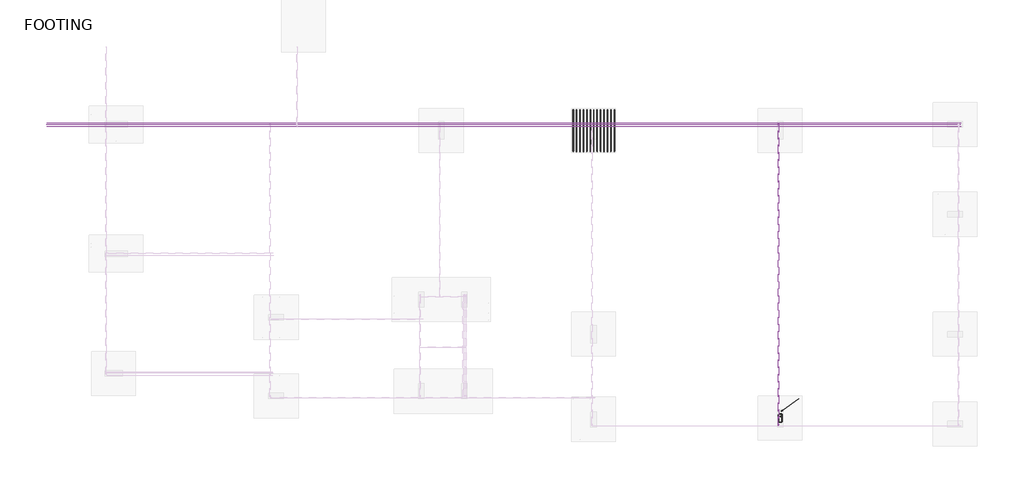
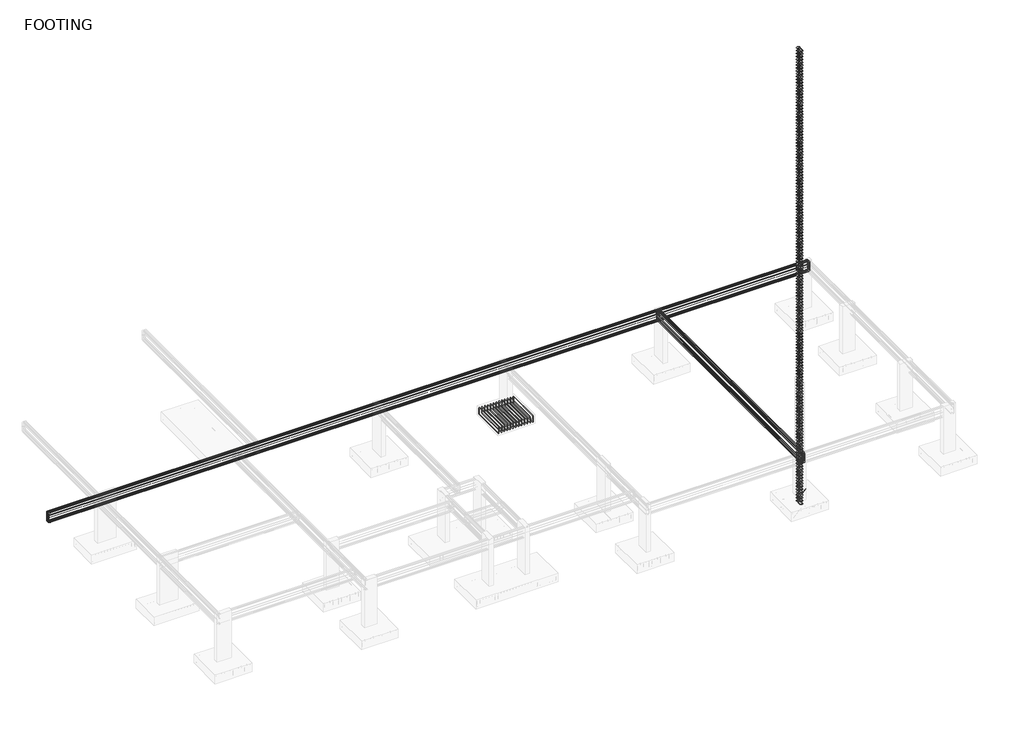
# One storey, part 7 of 12: 10 reinforcing bars.
"""IFC4 building model written with IfcOpenShell, lengths in millimetres."""

from ifc_helpers import new_model, si_unit, point, frame, origin, place, context, project, spatial, polyline, circle_curve, trimmed, segment, composite_curve, source, transform, mapped, element, save
from ifc_brep_helpers import swept_disk

model = new_model("IFC4")

# Units and contexts
model_context = context("Model", 3, world=origin())
ifc_project = project(units=[si_unit("LENGTHUNIT", "METRE", prefix="MILLI")], contexts=[model_context])

# Site, building, storey
site = spatial("IfcSite", under=ifc_project)
building = spatial("IfcBuilding", under=site)
storey = spatial("IfcBuildingStorey", under=building, Name="FOOTING", Elevation=-5638.8)

# Reinforcing bars
placement = place(None, origin())
reinforcing_bar_shape = source(origin(), model_context, "Body", "SolidModel", [
    swept_disk(composite_curve([segment(polyline([(5332.7998335, -3250.2541655, -5788.8), (5332.7998335, -3250.2541655, -5975.4)]), True, "CONTINUOUS"), segment(trimmed(circle_curve(frame((5332.7998335, -3194.8041655, -5975.4), z_axis=(1.0, 0.0, 0.0), x_axis=(0.0, -55.44999999999982, 0.0)), 55.45), [point((5332.7998335, -3250.2541655, -5975.4))], [point((5332.7998335, -3194.8041655, -6030.85))], True, "CARTESIAN"), True, "CONTINUOUS"), segment(polyline([(5332.7998335, -3194.8041655, -6030.85), (5332.7998335, -1621.6041655, -6030.85)]), True, "CONTINUOUS"), segment(trimmed(circle_curve(frame((5332.7998335, -1621.6041655, -5975.4), z_axis=(1.0, 0.0, 0.0), x_axis=(0.0, 0.0, -55.45000000000073)), 55.45), [point((5332.7998335, -1621.6041655, -6030.85))], [point((5332.7998335, -1566.1541655, -5975.4))], True, "CARTESIAN"), True, "CONTINUOUS"), segment(polyline([(5332.7998335, -1566.1541655, -5975.4), (5332.7998335, -1566.1541655, -5788.8)]), True, "CONTINUOUS")], self_intersect=False), 7.95),
])
element("IfcReinforcingBar", 1, at=placement, inside=storey, context=model_context, shape_type="MappedRepresentation", body=[
    mapped(reinforcing_bar_shape, transform((0.0, 0.0, 0.0), x_axis=(1.0, 0.0, 0.0), y_axis=(0.0, 1.0, 0.0), z_axis=(0.0, 0.0, 1.0))),
    mapped(reinforcing_bar_shape, transform((-140.3416667, 0.0, 0.0), x_axis=(1.0, 0.0, 0.0), y_axis=(0.0, 1.0, 0.0), z_axis=(0.0, 0.0, 1.0))),
    mapped(reinforcing_bar_shape, transform((-280.6833333, 0.0, 0.0), x_axis=(1.0, 0.0, 0.0), y_axis=(0.0, 1.0, 0.0), z_axis=(0.0, 0.0, 1.0))),
    mapped(reinforcing_bar_shape, transform((-421.025, 0.0, 0.0), x_axis=(1.0, 0.0, 0.0), y_axis=(0.0, 1.0, 0.0), z_axis=(0.0, 0.0, 1.0))),
    mapped(reinforcing_bar_shape, transform((-561.3666667, 0.0, 0.0), x_axis=(1.0, 0.0, 0.0), y_axis=(0.0, 1.0, 0.0), z_axis=(0.0, 0.0, 1.0))),
    mapped(reinforcing_bar_shape, transform((-701.7083333, 0.0, 0.0), x_axis=(1.0, 0.0, 0.0), y_axis=(0.0, 1.0, 0.0), z_axis=(0.0, 0.0, 1.0))),
    mapped(reinforcing_bar_shape, transform((-842.05, 0.0, 0.0), x_axis=(1.0, 0.0, 0.0), y_axis=(0.0, 1.0, 0.0), z_axis=(0.0, 0.0, 1.0))),
    mapped(reinforcing_bar_shape, transform((-982.3916667, 0.0, 0.0), x_axis=(1.0, 0.0, 0.0), y_axis=(0.0, 1.0, 0.0), z_axis=(0.0, 0.0, 1.0))),
    mapped(reinforcing_bar_shape, transform((-1122.7333333, 0.0, 0.0), x_axis=(1.0, 0.0, 0.0), y_axis=(0.0, 1.0, 0.0), z_axis=(0.0, 0.0, 1.0))),
    mapped(reinforcing_bar_shape, transform((-1263.075, 0.0, 0.0), x_axis=(1.0, 0.0, 0.0), y_axis=(0.0, 1.0, 0.0), z_axis=(0.0, 0.0, 1.0))),
    mapped(reinforcing_bar_shape, transform((-1403.4166667, 0.0, 0.0), x_axis=(1.0, 0.0, 0.0), y_axis=(0.0, 1.0, 0.0), z_axis=(0.0, 0.0, 1.0))),
    mapped(reinforcing_bar_shape, transform((-1543.7583333, 0.0, 0.0), x_axis=(1.0, 0.0, 0.0), y_axis=(0.0, 1.0, 0.0), z_axis=(0.0, 0.0, 1.0))),
    mapped(reinforcing_bar_shape, transform((-1684.1, 0.0, 0.0), x_axis=(1.0, 0.0, 0.0), y_axis=(0.0, 1.0, 0.0), z_axis=(0.0, 0.0, 1.0))),
])
reinforcing_bar_2_shape = source(origin(), model_context, "Body", "SolidModel", [
    swept_disk(composite_curve([segment(polyline([(5323.6597994, -1564.5541655, -5888.8), (5323.6597994, -1564.5541655, -5741.5)]), True, "CONTINUOUS"), segment(trimmed(circle_curve(frame((5323.6597994, -1610.9041655, -5741.5), z_axis=(1.0, 0.0, 0.0), x_axis=(0.0, 46.350000000000136, 0.0)), 46.35), [point((5323.6597994, -1564.5541655, -5741.5))], [point((5323.6597994, -1610.9041655, -5695.15))], True, "CARTESIAN"), True, "CONTINUOUS"), segment(polyline([(5323.6597994, -1610.9041655, -5695.15), (5323.6597994, -3205.5041655, -5695.15)]), True, "CONTINUOUS"), segment(trimmed(circle_curve(frame((5323.6597994, -3205.5041655, -5741.5), z_axis=(1.0, 0.0, 0.0), x_axis=(0.0, 0.0, 46.350000000000364)), 46.35), [point((5323.6597994, -3205.5041655, -5695.15))], [point((5323.6597994, -3251.8541655, -5741.5))], True, "CARTESIAN"), True, "CONTINUOUS"), segment(polyline([(5323.6597994, -3251.8541655, -5741.5), (5323.6597994, -3251.8541655, -5888.8)]), True, "CONTINUOUS")], self_intersect=False), 6.35),
])
element("IfcReinforcingBar", 2, at=placement, inside=storey, context=model_context, shape_type="MappedRepresentation", body=[
    mapped(reinforcing_bar_2_shape, transform((0.0, 0.0, 0.0), x_axis=(1.0, 0.0, 0.0), y_axis=(0.0, 1.0, 0.0), z_axis=(0.0, 0.0, 1.0))),
    mapped(reinforcing_bar_2_shape, transform((-138.4829293, 0.0, 0.0), x_axis=(1.0, 0.0, 0.0), y_axis=(0.0, 1.0, 0.0), z_axis=(0.0, 0.0, 1.0))),
    mapped(reinforcing_bar_2_shape, transform((-276.9658586, 0.0, 0.0), x_axis=(1.0, 0.0, 0.0), y_axis=(0.0, 1.0, 0.0), z_axis=(0.0, 0.0, 1.0))),
    mapped(reinforcing_bar_2_shape, transform((-415.4487879, 0.0, 0.0), x_axis=(1.0, 0.0, 0.0), y_axis=(0.0, 1.0, 0.0), z_axis=(0.0, 0.0, 1.0))),
    mapped(reinforcing_bar_2_shape, transform((-553.9317172, 0.0, 0.0), x_axis=(1.0, 0.0, 0.0), y_axis=(0.0, 1.0, 0.0), z_axis=(0.0, 0.0, 1.0))),
    mapped(reinforcing_bar_2_shape, transform((-692.4146465, 0.0, 0.0), x_axis=(1.0, 0.0, 0.0), y_axis=(0.0, 1.0, 0.0), z_axis=(0.0, 0.0, 1.0))),
    mapped(reinforcing_bar_2_shape, transform((-830.8975758, 0.0, 0.0), x_axis=(1.0, 0.0, 0.0), y_axis=(0.0, 1.0, 0.0), z_axis=(0.0, 0.0, 1.0))),
    mapped(reinforcing_bar_2_shape, transform((-969.3805051, 0.0, 0.0), x_axis=(1.0, 0.0, 0.0), y_axis=(0.0, 1.0, 0.0), z_axis=(0.0, 0.0, 1.0))),
    mapped(reinforcing_bar_2_shape, transform((-1107.8634344, 0.0, 0.0), x_axis=(1.0, 0.0, 0.0), y_axis=(0.0, 1.0, 0.0), z_axis=(0.0, 0.0, 1.0))),
    mapped(reinforcing_bar_2_shape, transform((-1246.3463637, 0.0, 0.0), x_axis=(1.0, 0.0, 0.0), y_axis=(0.0, 1.0, 0.0), z_axis=(0.0, 0.0, 1.0))),
    mapped(reinforcing_bar_2_shape, transform((-1384.8292929, 0.0, 0.0), x_axis=(1.0, 0.0, 0.0), y_axis=(0.0, 1.0, 0.0), z_axis=(0.0, 0.0, 1.0))),
    mapped(reinforcing_bar_2_shape, transform((-1523.3122222, 0.0, 0.0), x_axis=(1.0, 0.0, 0.0), y_axis=(0.0, 1.0, 0.0), z_axis=(0.0, 0.0, 1.0))),
    mapped(reinforcing_bar_2_shape, transform((-1661.7951515, 0.0, 0.0), x_axis=(1.0, 0.0, 0.0), y_axis=(0.0, 1.0, 0.0), z_axis=(0.0, 0.0, 1.0))),
])
element("IfcReinforcingBar", 3, at=placement, inside=storey, context=model_context, shape_type="SolidModel", body=[
    swept_disk(composite_curve([segment(polyline([(12139.6884899, -13823.5930989, 367.9679278), (12139.6884899, -13823.5930989, -5942.169349)]), True, "CONTINUOUS"), segment(trimmed(circle_curve(frame((12184.6874666, -13791.192565, -5942.169349), z_axis=(0.5843198177171824, -0.8115234750904984, 0.0), x_axis=(-44.99897670000064, -32.40053390000139, 0.0)), 55.45), [point((12139.6884899, -13823.5930989, -5942.169349))], [point((12184.6874666, -13791.192565, -5997.619349))], True, "CARTESIAN"), True, "CONTINUOUS"), segment(polyline([(12184.6874666, -13791.192565, -5997.619349), (12832.625225, -13324.6590827, -5997.619349)]), True, "CONTINUOUS")], self_intersect=False), 7.95),
])
reinforcing_bar_3_shape = source(origin(), model_context, "Body", "SolidModel", [
    swept_disk(composite_curve([segment(polyline([(12052.5484639, -13947.9700357, 17473.9463752), (12128.0484639, -13947.9700357, 17473.9463752)]), True, "CONTINUOUS"), segment(trimmed(circle_curve(frame((12128.0484639, -13972.7200357, 17473.9463752), z_axis=(0.0, 0.0, -1.0), x_axis=(0.0, 24.75, 0.0)), 24.75), [point((12128.0484639, -13947.9700357, 17473.9463752))], [point((12152.7984639, -13972.7200357, 17473.9463752))], True, "CARTESIAN"), True, "CONTINUOUS"), segment(polyline([(12152.7984639, -13972.7200357, 17473.9463752), (12152.7984639, -14257.5052311, 17473.9463752)]), True, "CONTINUOUS"), segment(trimmed(circle_curve(frame((12128.0484639, -14257.5052311, 17473.9463752), z_axis=(0.0, 0.0, -1.0), x_axis=(24.75, 0.0, 0.0)), 24.75), [point((12152.7984639, -14257.5052311, 17473.9463752))], [point((12128.0484639, -14282.2552311, 17473.9463752))], True, "CARTESIAN"), True, "CONTINUOUS"), segment(polyline([(12128.0484639, -14282.2552311, 17473.9463752), (12040.5498335, -14282.2552311, 17473.9463752)]), True, "CONTINUOUS"), segment(trimmed(circle_curve(frame((12040.5498335, -14257.5151345, 17474.64646), z_axis=(0.0, 0.028286253419373603, -0.99959986387929), x_axis=(0.0, -24.74009660000047, -0.7000847999988764)), 24.75), [point((12040.5498335, -14282.2552311, 17473.9463752))], [point((12015.7998335, -14257.5151345, 17474.64646))], True, "CARTESIAN"), True, "CONTINUOUS"), segment(polyline([(12015.7998335, -14257.5151345, 17474.64646), (12015.7998335, -13971.2775299, 17482.7462904)]), True, "CONTINUOUS"), segment(trimmed(circle_curve(frame((12040.5498335, -13971.2775299, 17482.7462904), z_axis=(0.0, 0.028286253419373603, -0.99959986387929), x_axis=(-24.75, 0.0, 0.0)), 24.75), [point((12015.7998335, -13971.2775299, 17482.7462904))], [point((12040.5498335, -13946.5374333, 17483.4463752))], True, "CARTESIAN"), True, "CONTINUOUS"), segment(polyline([(12040.5498335, -13946.5374333, 17483.4463752), (12130.1498335, -13946.5374333, 17483.4463752)]), True, "CONTINUOUS"), segment(trimmed(circle_curve(frame((12130.1498335, -13971.2874333, 17483.4463752), z_axis=(0.0, 0.0, -1.0), x_axis=(0.0, 24.75, 0.0)), 24.75), [point((12130.1498335, -13946.5374333, 17483.4463752))], [point((12147.6507263, -13988.7883261, 17483.4463752))], True, "CARTESIAN"), True, "CONTINUOUS"), segment(polyline([(12147.6507263, -13988.7883261, 17483.4463752), (12090.2448376, -14046.1942149, 17483.4463752)]), True, "CONTINUOUS")], self_intersect=False), 4.75),
])
element("IfcReinforcingBar", 4, at=placement, inside=storey, context=model_context, shape_type="MappedRepresentation", body=[
    mapped(reinforcing_bar_3_shape, transform((0.0, 0.0, 0.0), x_axis=(1.0, 0.0, 0.0), y_axis=(0.0, 1.0, 0.0), z_axis=(0.0, 0.0, 1.0))),
    mapped(reinforcing_bar_3_shape, transform((0.0, 0.0, -149.1260916), x_axis=(1.0, 0.0, 0.0), y_axis=(0.0, 1.0, 0.0), z_axis=(0.0, 0.0, 1.0))),
    mapped(reinforcing_bar_3_shape, transform((0.0, 0.0, -298.2521831), x_axis=(1.0, 0.0, 0.0), y_axis=(0.0, 1.0, 0.0), z_axis=(0.0, 0.0, 1.0))),
    mapped(reinforcing_bar_3_shape, transform((0.0, 0.0, -447.3782747), x_axis=(1.0, 0.0, 0.0), y_axis=(0.0, 1.0, 0.0), z_axis=(0.0, 0.0, 1.0))),
    mapped(reinforcing_bar_3_shape, transform((0.0, 0.0, -596.5043662), x_axis=(1.0, 0.0, 0.0), y_axis=(0.0, 1.0, 0.0), z_axis=(0.0, 0.0, 1.0))),
    mapped(reinforcing_bar_3_shape, transform((0.0, 0.0, -745.6304578), x_axis=(1.0, 0.0, 0.0), y_axis=(0.0, 1.0, 0.0), z_axis=(0.0, 0.0, 1.0))),
    mapped(reinforcing_bar_3_shape, transform((0.0, 0.0, -894.7565494), x_axis=(1.0, 0.0, 0.0), y_axis=(0.0, 1.0, 0.0), z_axis=(0.0, 0.0, 1.0))),
    mapped(reinforcing_bar_3_shape, transform((0.0, 0.0, -1043.8826409), x_axis=(1.0, 0.0, 0.0), y_axis=(0.0, 1.0, 0.0), z_axis=(0.0, 0.0, 1.0))),
    mapped(reinforcing_bar_3_shape, transform((0.0, 0.0, -1193.0087325), x_axis=(1.0, 0.0, 0.0), y_axis=(0.0, 1.0, 0.0), z_axis=(0.0, 0.0, 1.0))),
    mapped(reinforcing_bar_3_shape, transform((0.0, 0.0, -1342.1348241), x_axis=(1.0, 0.0, 0.0), y_axis=(0.0, 1.0, 0.0), z_axis=(0.0, 0.0, 1.0))),
    mapped(reinforcing_bar_3_shape, transform((0.0, 0.0, -1491.2609156), x_axis=(1.0, 0.0, 0.0), y_axis=(0.0, 1.0, 0.0), z_axis=(0.0, 0.0, 1.0))),
    mapped(reinforcing_bar_3_shape, transform((0.0, 0.0, -1640.3870072), x_axis=(1.0, 0.0, 0.0), y_axis=(0.0, 1.0, 0.0), z_axis=(0.0, 0.0, 1.0))),
    mapped(reinforcing_bar_3_shape, transform((0.0, 0.0, -1789.5130987), x_axis=(1.0, 0.0, 0.0), y_axis=(0.0, 1.0, 0.0), z_axis=(0.0, 0.0, 1.0))),
    mapped(reinforcing_bar_3_shape, transform((0.0, 0.0, -1938.6391903), x_axis=(1.0, 0.0, 0.0), y_axis=(0.0, 1.0, 0.0), z_axis=(0.0, 0.0, 1.0))),
    mapped(reinforcing_bar_3_shape, transform((0.0, 0.0, -2087.7652819), x_axis=(1.0, 0.0, 0.0), y_axis=(0.0, 1.0, 0.0), z_axis=(0.0, 0.0, 1.0))),
    mapped(reinforcing_bar_3_shape, transform((0.0, 0.0, -2236.8913734), x_axis=(1.0, 0.0, 0.0), y_axis=(0.0, 1.0, 0.0), z_axis=(0.0, 0.0, 1.0))),
    mapped(reinforcing_bar_3_shape, transform((0.0, 0.0, -2386.017465), x_axis=(1.0, 0.0, 0.0), y_axis=(0.0, 1.0, 0.0), z_axis=(0.0, 0.0, 1.0))),
    mapped(reinforcing_bar_3_shape, transform((0.0, 0.0, -2535.1435566), x_axis=(1.0, 0.0, 0.0), y_axis=(0.0, 1.0, 0.0), z_axis=(0.0, 0.0, 1.0))),
    mapped(reinforcing_bar_3_shape, transform((0.0, 0.0, -2684.2696481), x_axis=(1.0, 0.0, 0.0), y_axis=(0.0, 1.0, 0.0), z_axis=(0.0, 0.0, 1.0))),
    mapped(reinforcing_bar_3_shape, transform((0.0, 0.0, -2833.3957397), x_axis=(1.0, 0.0, 0.0), y_axis=(0.0, 1.0, 0.0), z_axis=(0.0, 0.0, 1.0))),
    mapped(reinforcing_bar_3_shape, transform((0.0, 0.0, -2982.5218312), x_axis=(1.0, 0.0, 0.0), y_axis=(0.0, 1.0, 0.0), z_axis=(0.0, 0.0, 1.0))),
    mapped(reinforcing_bar_3_shape, transform((0.0, 0.0, -3131.6479228), x_axis=(1.0, 0.0, 0.0), y_axis=(0.0, 1.0, 0.0), z_axis=(0.0, 0.0, 1.0))),
    mapped(reinforcing_bar_3_shape, transform((0.0, 0.0, -3280.7740144), x_axis=(1.0, 0.0, 0.0), y_axis=(0.0, 1.0, 0.0), z_axis=(0.0, 0.0, 1.0))),
    mapped(reinforcing_bar_3_shape, transform((0.0, 0.0, -3429.9001059), x_axis=(1.0, 0.0, 0.0), y_axis=(0.0, 1.0, 0.0), z_axis=(0.0, 0.0, 1.0))),
    mapped(reinforcing_bar_3_shape, transform((0.0, 0.0, -3579.0261975), x_axis=(1.0, 0.0, 0.0), y_axis=(0.0, 1.0, 0.0), z_axis=(0.0, 0.0, 1.0))),
    mapped(reinforcing_bar_3_shape, transform((0.0, 0.0, -3728.152289), x_axis=(1.0, 0.0, 0.0), y_axis=(0.0, 1.0, 0.0), z_axis=(0.0, 0.0, 1.0))),
    mapped(reinforcing_bar_3_shape, transform((0.0, 0.0, -3877.2783806), x_axis=(1.0, 0.0, 0.0), y_axis=(0.0, 1.0, 0.0), z_axis=(0.0, 0.0, 1.0))),
    mapped(reinforcing_bar_3_shape, transform((0.0, 0.0, -4026.4044722), x_axis=(1.0, 0.0, 0.0), y_axis=(0.0, 1.0, 0.0), z_axis=(0.0, 0.0, 1.0))),
    mapped(reinforcing_bar_3_shape, transform((0.0, 0.0, -4175.5305637), x_axis=(1.0, 0.0, 0.0), y_axis=(0.0, 1.0, 0.0), z_axis=(0.0, 0.0, 1.0))),
    mapped(reinforcing_bar_3_shape, transform((0.0, 0.0, -4324.6566553), x_axis=(1.0, 0.0, 0.0), y_axis=(0.0, 1.0, 0.0), z_axis=(0.0, 0.0, 1.0))),
    mapped(reinforcing_bar_3_shape, transform((0.0, 0.0, -4473.7827469), x_axis=(1.0, 0.0, 0.0), y_axis=(0.0, 1.0, 0.0), z_axis=(0.0, 0.0, 1.0))),
    mapped(reinforcing_bar_3_shape, transform((0.0, 0.0, -4622.9088384), x_axis=(1.0, 0.0, 0.0), y_axis=(0.0, 1.0, 0.0), z_axis=(0.0, 0.0, 1.0))),
    mapped(reinforcing_bar_3_shape, transform((0.0, 0.0, -4772.03493), x_axis=(1.0, 0.0, 0.0), y_axis=(0.0, 1.0, 0.0), z_axis=(0.0, 0.0, 1.0))),
    mapped(reinforcing_bar_3_shape, transform((0.0, 0.0, -4921.1610215), x_axis=(1.0, 0.0, 0.0), y_axis=(0.0, 1.0, 0.0), z_axis=(0.0, 0.0, 1.0))),
    mapped(reinforcing_bar_3_shape, transform((0.0, 0.0, -5070.2871131), x_axis=(1.0, 0.0, 0.0), y_axis=(0.0, 1.0, 0.0), z_axis=(0.0, 0.0, 1.0))),
    mapped(reinforcing_bar_3_shape, transform((0.0, 0.0, -5219.4132047), x_axis=(1.0, 0.0, 0.0), y_axis=(0.0, 1.0, 0.0), z_axis=(0.0, 0.0, 1.0))),
    mapped(reinforcing_bar_3_shape, transform((0.0, 0.0, -5368.5392962), x_axis=(1.0, 0.0, 0.0), y_axis=(0.0, 1.0, 0.0), z_axis=(0.0, 0.0, 1.0))),
    mapped(reinforcing_bar_3_shape, transform((0.0, 0.0, -5517.6653878), x_axis=(1.0, 0.0, 0.0), y_axis=(0.0, 1.0, 0.0), z_axis=(0.0, 0.0, 1.0))),
    mapped(reinforcing_bar_3_shape, transform((0.0, 0.0, -5666.7914793), x_axis=(1.0, 0.0, 0.0), y_axis=(0.0, 1.0, 0.0), z_axis=(0.0, 0.0, 1.0))),
    mapped(reinforcing_bar_3_shape, transform((0.0, 0.0, -5815.9175709), x_axis=(1.0, 0.0, 0.0), y_axis=(0.0, 1.0, 0.0), z_axis=(0.0, 0.0, 1.0))),
    mapped(reinforcing_bar_3_shape, transform((0.0, 0.0, -5965.0436625), x_axis=(1.0, 0.0, 0.0), y_axis=(0.0, 1.0, 0.0), z_axis=(0.0, 0.0, 1.0))),
    mapped(reinforcing_bar_3_shape, transform((0.0, 0.0, -6114.169754), x_axis=(1.0, 0.0, 0.0), y_axis=(0.0, 1.0, 0.0), z_axis=(0.0, 0.0, 1.0))),
    mapped(reinforcing_bar_3_shape, transform((0.0, 0.0, -6263.2958456), x_axis=(1.0, 0.0, 0.0), y_axis=(0.0, 1.0, 0.0), z_axis=(0.0, 0.0, 1.0))),
    mapped(reinforcing_bar_3_shape, transform((0.0, 0.0, -6412.4219372), x_axis=(1.0, 0.0, 0.0), y_axis=(0.0, 1.0, 0.0), z_axis=(0.0, 0.0, 1.0))),
    mapped(reinforcing_bar_3_shape, transform((0.0, 0.0, -6561.5480287), x_axis=(1.0, 0.0, 0.0), y_axis=(0.0, 1.0, 0.0), z_axis=(0.0, 0.0, 1.0))),
    mapped(reinforcing_bar_3_shape, transform((0.0, 0.0, -6710.6741203), x_axis=(1.0, 0.0, 0.0), y_axis=(0.0, 1.0, 0.0), z_axis=(0.0, 0.0, 1.0))),
    mapped(reinforcing_bar_3_shape, transform((0.0, 0.0, -6859.8002118), x_axis=(1.0, 0.0, 0.0), y_axis=(0.0, 1.0, 0.0), z_axis=(0.0, 0.0, 1.0))),
    mapped(reinforcing_bar_3_shape, transform((0.0, 0.0, -7008.9263034), x_axis=(1.0, 0.0, 0.0), y_axis=(0.0, 1.0, 0.0), z_axis=(0.0, 0.0, 1.0))),
    mapped(reinforcing_bar_3_shape, transform((0.0, 0.0, -7158.052395), x_axis=(1.0, 0.0, 0.0), y_axis=(0.0, 1.0, 0.0), z_axis=(0.0, 0.0, 1.0))),
    mapped(reinforcing_bar_3_shape, transform((0.0, 0.0, -7307.1784865), x_axis=(1.0, 0.0, 0.0), y_axis=(0.0, 1.0, 0.0), z_axis=(0.0, 0.0, 1.0))),
    mapped(reinforcing_bar_3_shape, transform((0.0, 0.0, -7456.3045781), x_axis=(1.0, 0.0, 0.0), y_axis=(0.0, 1.0, 0.0), z_axis=(0.0, 0.0, 1.0))),
    mapped(reinforcing_bar_3_shape, transform((0.0, 0.0, -7605.4306697), x_axis=(1.0, 0.0, 0.0), y_axis=(0.0, 1.0, 0.0), z_axis=(0.0, 0.0, 1.0))),
    mapped(reinforcing_bar_3_shape, transform((0.0, 0.0, -7754.5567612), x_axis=(1.0, 0.0, 0.0), y_axis=(0.0, 1.0, 0.0), z_axis=(0.0, 0.0, 1.0))),
    mapped(reinforcing_bar_3_shape, transform((0.0, 0.0, -7903.6828528), x_axis=(1.0, 0.0, 0.0), y_axis=(0.0, 1.0, 0.0), z_axis=(0.0, 0.0, 1.0))),
    mapped(reinforcing_bar_3_shape, transform((0.0, 0.0, -8052.8089443), x_axis=(1.0, 0.0, 0.0), y_axis=(0.0, 1.0, 0.0), z_axis=(0.0, 0.0, 1.0))),
    mapped(reinforcing_bar_3_shape, transform((0.0, 0.0, -8201.9350359), x_axis=(1.0, 0.0, 0.0), y_axis=(0.0, 1.0, 0.0), z_axis=(0.0, 0.0, 1.0))),
    mapped(reinforcing_bar_3_shape, transform((0.0, 0.0, -8351.0611275), x_axis=(1.0, 0.0, 0.0), y_axis=(0.0, 1.0, 0.0), z_axis=(0.0, 0.0, 1.0))),
    mapped(reinforcing_bar_3_shape, transform((0.0, 0.0, -8500.187219), x_axis=(1.0, 0.0, 0.0), y_axis=(0.0, 1.0, 0.0), z_axis=(0.0, 0.0, 1.0))),
    mapped(reinforcing_bar_3_shape, transform((0.0, 0.0, -8649.3133106), x_axis=(1.0, 0.0, 0.0), y_axis=(0.0, 1.0, 0.0), z_axis=(0.0, 0.0, 1.0))),
    mapped(reinforcing_bar_3_shape, transform((0.0, 0.0, -8798.4394021), x_axis=(1.0, 0.0, 0.0), y_axis=(0.0, 1.0, 0.0), z_axis=(0.0, 0.0, 1.0))),
    mapped(reinforcing_bar_3_shape, transform((0.0, 0.0, -8947.5654937), x_axis=(1.0, 0.0, 0.0), y_axis=(0.0, 1.0, 0.0), z_axis=(0.0, 0.0, 1.0))),
    mapped(reinforcing_bar_3_shape, transform((0.0, 0.0, -9096.6915853), x_axis=(1.0, 0.0, 0.0), y_axis=(0.0, 1.0, 0.0), z_axis=(0.0, 0.0, 1.0))),
    mapped(reinforcing_bar_3_shape, transform((0.0, 0.0, -9245.8176768), x_axis=(1.0, 0.0, 0.0), y_axis=(0.0, 1.0, 0.0), z_axis=(0.0, 0.0, 1.0))),
    mapped(reinforcing_bar_3_shape, transform((0.0, 0.0, -9394.9437684), x_axis=(1.0, 0.0, 0.0), y_axis=(0.0, 1.0, 0.0), z_axis=(0.0, 0.0, 1.0))),
    mapped(reinforcing_bar_3_shape, transform((0.0, 0.0, -9544.06986), x_axis=(1.0, 0.0, 0.0), y_axis=(0.0, 1.0, 0.0), z_axis=(0.0, 0.0, 1.0))),
    mapped(reinforcing_bar_3_shape, transform((0.0, 0.0, -9693.1959515), x_axis=(1.0, 0.0, 0.0), y_axis=(0.0, 1.0, 0.0), z_axis=(0.0, 0.0, 1.0))),
    mapped(reinforcing_bar_3_shape, transform((0.0, 0.0, -9842.3220431), x_axis=(1.0, 0.0, 0.0), y_axis=(0.0, 1.0, 0.0), z_axis=(0.0, 0.0, 1.0))),
    mapped(reinforcing_bar_3_shape, transform((0.0, 0.0, -9991.4481346), x_axis=(1.0, 0.0, 0.0), y_axis=(0.0, 1.0, 0.0), z_axis=(0.0, 0.0, 1.0))),
    mapped(reinforcing_bar_3_shape, transform((0.0, 0.0, -10140.5742262), x_axis=(1.0, 0.0, 0.0), y_axis=(0.0, 1.0, 0.0), z_axis=(0.0, 0.0, 1.0))),
    mapped(reinforcing_bar_3_shape, transform((0.0, 0.0, -10289.7003178), x_axis=(1.0, 0.0, 0.0), y_axis=(0.0, 1.0, 0.0), z_axis=(0.0, 0.0, 1.0))),
    mapped(reinforcing_bar_3_shape, transform((0.0, 0.0, -10438.8264093), x_axis=(1.0, 0.0, 0.0), y_axis=(0.0, 1.0, 0.0), z_axis=(0.0, 0.0, 1.0))),
    mapped(reinforcing_bar_3_shape, transform((0.0, 0.0, -10587.9525009), x_axis=(1.0, 0.0, 0.0), y_axis=(0.0, 1.0, 0.0), z_axis=(0.0, 0.0, 1.0))),
    mapped(reinforcing_bar_3_shape, transform((0.0, 0.0, -10737.0785924), x_axis=(1.0, 0.0, 0.0), y_axis=(0.0, 1.0, 0.0), z_axis=(0.0, 0.0, 1.0))),
    mapped(reinforcing_bar_3_shape, transform((0.0, 0.0, -10886.204684), x_axis=(1.0, 0.0, 0.0), y_axis=(0.0, 1.0, 0.0), z_axis=(0.0, 0.0, 1.0))),
    mapped(reinforcing_bar_3_shape, transform((0.0, 0.0, -11035.3307756), x_axis=(1.0, 0.0, 0.0), y_axis=(0.0, 1.0, 0.0), z_axis=(0.0, 0.0, 1.0))),
    mapped(reinforcing_bar_3_shape, transform((0.0, 0.0, -11184.4568671), x_axis=(1.0, 0.0, 0.0), y_axis=(0.0, 1.0, 0.0), z_axis=(0.0, 0.0, 1.0))),
    mapped(reinforcing_bar_3_shape, transform((0.0, 0.0, -11333.5829587), x_axis=(1.0, 0.0, 0.0), y_axis=(0.0, 1.0, 0.0), z_axis=(0.0, 0.0, 1.0))),
    mapped(reinforcing_bar_3_shape, transform((0.0, 0.0, -11482.7090503), x_axis=(1.0, 0.0, 0.0), y_axis=(0.0, 1.0, 0.0), z_axis=(0.0, 0.0, 1.0))),
    mapped(reinforcing_bar_3_shape, transform((0.0, 0.0, -11631.8351418), x_axis=(1.0, 0.0, 0.0), y_axis=(0.0, 1.0, 0.0), z_axis=(0.0, 0.0, 1.0))),
    mapped(reinforcing_bar_3_shape, transform((0.0, 0.0, -11780.9612334), x_axis=(1.0, 0.0, 0.0), y_axis=(0.0, 1.0, 0.0), z_axis=(0.0, 0.0, 1.0))),
    mapped(reinforcing_bar_3_shape, transform((0.0, 0.0, -11930.0873249), x_axis=(1.0, 0.0, 0.0), y_axis=(0.0, 1.0, 0.0), z_axis=(0.0, 0.0, 1.0))),
    mapped(reinforcing_bar_3_shape, transform((0.0, 0.0, -12079.2134165), x_axis=(1.0, 0.0, 0.0), y_axis=(0.0, 1.0, 0.0), z_axis=(0.0, 0.0, 1.0))),
    mapped(reinforcing_bar_3_shape, transform((0.0, 0.0, -12228.3395081), x_axis=(1.0, 0.0, 0.0), y_axis=(0.0, 1.0, 0.0), z_axis=(0.0, 0.0, 1.0))),
    mapped(reinforcing_bar_3_shape, transform((0.0, 0.0, -12377.4655996), x_axis=(1.0, 0.0, 0.0), y_axis=(0.0, 1.0, 0.0), z_axis=(0.0, 0.0, 1.0))),
    mapped(reinforcing_bar_3_shape, transform((0.0, 0.0, -12526.5916912), x_axis=(1.0, 0.0, 0.0), y_axis=(0.0, 1.0, 0.0), z_axis=(0.0, 0.0, 1.0))),
    mapped(reinforcing_bar_3_shape, transform((0.0, 0.0, -12675.7177828), x_axis=(1.0, 0.0, 0.0), y_axis=(0.0, 1.0, 0.0), z_axis=(0.0, 0.0, 1.0))),
    mapped(reinforcing_bar_3_shape, transform((0.0, 0.0, -12824.8438743), x_axis=(1.0, 0.0, 0.0), y_axis=(0.0, 1.0, 0.0), z_axis=(0.0, 0.0, 1.0))),
    mapped(reinforcing_bar_3_shape, transform((0.0, 0.0, -12973.9699659), x_axis=(1.0, 0.0, 0.0), y_axis=(0.0, 1.0, 0.0), z_axis=(0.0, 0.0, 1.0))),
    mapped(reinforcing_bar_3_shape, transform((0.0, 0.0, -13123.0960574), x_axis=(1.0, 0.0, 0.0), y_axis=(0.0, 1.0, 0.0), z_axis=(0.0, 0.0, 1.0))),
    mapped(reinforcing_bar_3_shape, transform((0.0, 0.0, -13272.222149), x_axis=(1.0, 0.0, 0.0), y_axis=(0.0, 1.0, 0.0), z_axis=(0.0, 0.0, 1.0))),
    mapped(reinforcing_bar_3_shape, transform((0.0, 0.0, -13421.3482406), x_axis=(1.0, 0.0, 0.0), y_axis=(0.0, 1.0, 0.0), z_axis=(0.0, 0.0, 1.0))),
    mapped(reinforcing_bar_3_shape, transform((0.0, 0.0, -13570.4743321), x_axis=(1.0, 0.0, 0.0), y_axis=(0.0, 1.0, 0.0), z_axis=(0.0, 0.0, 1.0))),
    mapped(reinforcing_bar_3_shape, transform((0.0, 0.0, -13719.6004237), x_axis=(1.0, 0.0, 0.0), y_axis=(0.0, 1.0, 0.0), z_axis=(0.0, 0.0, 1.0))),
    mapped(reinforcing_bar_3_shape, transform((0.0, 0.0, -13868.7265152), x_axis=(1.0, 0.0, 0.0), y_axis=(0.0, 1.0, 0.0), z_axis=(0.0, 0.0, 1.0))),
    mapped(reinforcing_bar_3_shape, transform((0.0, 0.0, -14017.8526068), x_axis=(1.0, 0.0, 0.0), y_axis=(0.0, 1.0, 0.0), z_axis=(0.0, 0.0, 1.0))),
    mapped(reinforcing_bar_3_shape, transform((0.0, 0.0, -14166.9786984), x_axis=(1.0, 0.0, 0.0), y_axis=(0.0, 1.0, 0.0), z_axis=(0.0, 0.0, 1.0))),
    mapped(reinforcing_bar_3_shape, transform((0.0, 0.0, -14316.1047899), x_axis=(1.0, 0.0, 0.0), y_axis=(0.0, 1.0, 0.0), z_axis=(0.0, 0.0, 1.0))),
    mapped(reinforcing_bar_3_shape, transform((0.0, 0.0, -14465.2308815), x_axis=(1.0, 0.0, 0.0), y_axis=(0.0, 1.0, 0.0), z_axis=(0.0, 0.0, 1.0))),
    mapped(reinforcing_bar_3_shape, transform((0.0, 0.0, -14614.3569731), x_axis=(1.0, 0.0, 0.0), y_axis=(0.0, 1.0, 0.0), z_axis=(0.0, 0.0, 1.0))),
    mapped(reinforcing_bar_3_shape, transform((0.0, 0.0, -14763.4830646), x_axis=(1.0, 0.0, 0.0), y_axis=(0.0, 1.0, 0.0), z_axis=(0.0, 0.0, 1.0))),
    mapped(reinforcing_bar_3_shape, transform((0.0, 0.0, -14912.6091562), x_axis=(1.0, 0.0, 0.0), y_axis=(0.0, 1.0, 0.0), z_axis=(0.0, 0.0, 1.0))),
    mapped(reinforcing_bar_3_shape, transform((0.0, 0.0, -15061.7352477), x_axis=(1.0, 0.0, 0.0), y_axis=(0.0, 1.0, 0.0), z_axis=(0.0, 0.0, 1.0))),
    mapped(reinforcing_bar_3_shape, transform((0.0, 0.0, -15210.8613393), x_axis=(1.0, 0.0, 0.0), y_axis=(0.0, 1.0, 0.0), z_axis=(0.0, 0.0, 1.0))),
    mapped(reinforcing_bar_3_shape, transform((0.0, 0.0, -15359.9874309), x_axis=(1.0, 0.0, 0.0), y_axis=(0.0, 1.0, 0.0), z_axis=(0.0, 0.0, 1.0))),
    mapped(reinforcing_bar_3_shape, transform((0.0, 0.0, -15509.1135224), x_axis=(1.0, 0.0, 0.0), y_axis=(0.0, 1.0, 0.0), z_axis=(0.0, 0.0, 1.0))),
    mapped(reinforcing_bar_3_shape, transform((0.0, 0.0, -15658.239614), x_axis=(1.0, 0.0, 0.0), y_axis=(0.0, 1.0, 0.0), z_axis=(0.0, 0.0, 1.0))),
    mapped(reinforcing_bar_3_shape, transform((0.0, 0.0, -15807.3657055), x_axis=(1.0, 0.0, 0.0), y_axis=(0.0, 1.0, 0.0), z_axis=(0.0, 0.0, 1.0))),
    mapped(reinforcing_bar_3_shape, transform((0.0, 0.0, -15956.4917971), x_axis=(1.0, 0.0, 0.0), y_axis=(0.0, 1.0, 0.0), z_axis=(0.0, 0.0, 1.0))),
    mapped(reinforcing_bar_3_shape, transform((0.0, 0.0, -16105.6178887), x_axis=(1.0, 0.0, 0.0), y_axis=(0.0, 1.0, 0.0), z_axis=(0.0, 0.0, 1.0))),
    mapped(reinforcing_bar_3_shape, transform((0.0, 0.0, -16254.7439802), x_axis=(1.0, 0.0, 0.0), y_axis=(0.0, 1.0, 0.0), z_axis=(0.0, 0.0, 1.0))),
    mapped(reinforcing_bar_3_shape, transform((0.0, 0.0, -16403.8700718), x_axis=(1.0, 0.0, 0.0), y_axis=(0.0, 1.0, 0.0), z_axis=(0.0, 0.0, 1.0))),
    mapped(reinforcing_bar_3_shape, transform((0.0, 0.0, -16552.9961634), x_axis=(1.0, 0.0, 0.0), y_axis=(0.0, 1.0, 0.0), z_axis=(0.0, 0.0, 1.0))),
    mapped(reinforcing_bar_3_shape, transform((0.0, 0.0, -16702.1222549), x_axis=(1.0, 0.0, 0.0), y_axis=(0.0, 1.0, 0.0), z_axis=(0.0, 0.0, 1.0))),
    mapped(reinforcing_bar_3_shape, transform((0.0, 0.0, -16851.2483465), x_axis=(1.0, 0.0, 0.0), y_axis=(0.0, 1.0, 0.0), z_axis=(0.0, 0.0, 1.0))),
    mapped(reinforcing_bar_3_shape, transform((0.0, 0.0, -17000.374438), x_axis=(1.0, 0.0, 0.0), y_axis=(0.0, 1.0, 0.0), z_axis=(0.0, 0.0, 1.0))),
    mapped(reinforcing_bar_3_shape, transform((0.0, 0.0, -17149.5005296), x_axis=(1.0, 0.0, 0.0), y_axis=(0.0, 1.0, 0.0), z_axis=(0.0, 0.0, 1.0))),
    mapped(reinforcing_bar_3_shape, transform((0.0, 0.0, -17298.6266212), x_axis=(1.0, 0.0, 0.0), y_axis=(0.0, 1.0, 0.0), z_axis=(0.0, 0.0, 1.0))),
    mapped(reinforcing_bar_3_shape, transform((0.0, 0.0, -17447.7527127), x_axis=(1.0, 0.0, 0.0), y_axis=(0.0, 1.0, 0.0), z_axis=(0.0, 0.0, 1.0))),
    mapped(reinforcing_bar_3_shape, transform((0.0, 0.0, -17596.8788043), x_axis=(1.0, 0.0, 0.0), y_axis=(0.0, 1.0, 0.0), z_axis=(0.0, 0.0, 1.0))),
    mapped(reinforcing_bar_3_shape, transform((0.0, 0.0, -17746.0048959), x_axis=(1.0, 0.0, 0.0), y_axis=(0.0, 1.0, 0.0), z_axis=(0.0, 0.0, 1.0))),
    mapped(reinforcing_bar_3_shape, transform((0.0, 0.0, -17895.1309874), x_axis=(1.0, 0.0, 0.0), y_axis=(0.0, 1.0, 0.0), z_axis=(0.0, 0.0, 1.0))),
    mapped(reinforcing_bar_3_shape, transform((0.0, 0.0, -18044.257079), x_axis=(1.0, 0.0, 0.0), y_axis=(0.0, 1.0, 0.0), z_axis=(0.0, 0.0, 1.0))),
    mapped(reinforcing_bar_3_shape, transform((0.0, 0.0, -18193.3831705), x_axis=(1.0, 0.0, 0.0), y_axis=(0.0, 1.0, 0.0), z_axis=(0.0, 0.0, 1.0))),
    mapped(reinforcing_bar_3_shape, transform((0.0, 0.0, -18342.5092621), x_axis=(1.0, 0.0, 0.0), y_axis=(0.0, 1.0, 0.0), z_axis=(0.0, 0.0, 1.0))),
    mapped(reinforcing_bar_3_shape, transform((0.0, 0.0, -18491.6353537), x_axis=(1.0, 0.0, 0.0), y_axis=(0.0, 1.0, 0.0), z_axis=(0.0, 0.0, 1.0))),
    mapped(reinforcing_bar_3_shape, transform((0.0, 0.0, -18640.7614452), x_axis=(1.0, 0.0, 0.0), y_axis=(0.0, 1.0, 0.0), z_axis=(0.0, 0.0, 1.0))),
    mapped(reinforcing_bar_3_shape, transform((0.0, 0.0, -18789.8875368), x_axis=(1.0, 0.0, 0.0), y_axis=(0.0, 1.0, 0.0), z_axis=(0.0, 0.0, 1.0))),
    mapped(reinforcing_bar_3_shape, transform((0.0, 0.0, -18939.0136283), x_axis=(1.0, 0.0, 0.0), y_axis=(0.0, 1.0, 0.0), z_axis=(0.0, 0.0, 1.0))),
    mapped(reinforcing_bar_3_shape, transform((0.0, 0.0, -19088.1397199), x_axis=(1.0, 0.0, 0.0), y_axis=(0.0, 1.0, 0.0), z_axis=(0.0, 0.0, 1.0))),
    mapped(reinforcing_bar_3_shape, transform((0.0, 0.0, -19237.2658115), x_axis=(1.0, 0.0, 0.0), y_axis=(0.0, 1.0, 0.0), z_axis=(0.0, 0.0, 1.0))),
    mapped(reinforcing_bar_3_shape, transform((0.0, 0.0, -19386.391903), x_axis=(1.0, 0.0, 0.0), y_axis=(0.0, 1.0, 0.0), z_axis=(0.0, 0.0, 1.0))),
    mapped(reinforcing_bar_3_shape, transform((0.0, 0.0, -19535.5179946), x_axis=(1.0, 0.0, 0.0), y_axis=(0.0, 1.0, 0.0), z_axis=(0.0, 0.0, 1.0))),
    mapped(reinforcing_bar_3_shape, transform((0.0, 0.0, -19684.6440862), x_axis=(1.0, 0.0, 0.0), y_axis=(0.0, 1.0, 0.0), z_axis=(0.0, 0.0, 1.0))),
    mapped(reinforcing_bar_3_shape, transform((0.0, 0.0, -19833.7701777), x_axis=(1.0, 0.0, 0.0), y_axis=(0.0, 1.0, 0.0), z_axis=(0.0, 0.0, 1.0))),
    mapped(reinforcing_bar_3_shape, transform((0.0, 0.0, -19982.8962693), x_axis=(1.0, 0.0, 0.0), y_axis=(0.0, 1.0, 0.0), z_axis=(0.0, 0.0, 1.0))),
    mapped(reinforcing_bar_3_shape, transform((0.0, 0.0, -20132.0223608), x_axis=(1.0, 0.0, 0.0), y_axis=(0.0, 1.0, 0.0), z_axis=(0.0, 0.0, 1.0))),
    mapped(reinforcing_bar_3_shape, transform((0.0, 0.0, -20281.1484524), x_axis=(1.0, 0.0, 0.0), y_axis=(0.0, 1.0, 0.0), z_axis=(0.0, 0.0, 1.0))),
    mapped(reinforcing_bar_3_shape, transform((0.0, 0.0, -20430.274544), x_axis=(1.0, 0.0, 0.0), y_axis=(0.0, 1.0, 0.0), z_axis=(0.0, 0.0, 1.0))),
    mapped(reinforcing_bar_3_shape, transform((0.0, 0.0, -20579.4006355), x_axis=(1.0, 0.0, 0.0), y_axis=(0.0, 1.0, 0.0), z_axis=(0.0, 0.0, 1.0))),
    mapped(reinforcing_bar_3_shape, transform((0.0, 0.0, -20728.5267271), x_axis=(1.0, 0.0, 0.0), y_axis=(0.0, 1.0, 0.0), z_axis=(0.0, 0.0, 1.0))),
    mapped(reinforcing_bar_3_shape, transform((0.0, 0.0, -20877.6528186), x_axis=(1.0, 0.0, 0.0), y_axis=(0.0, 1.0, 0.0), z_axis=(0.0, 0.0, 1.0))),
    mapped(reinforcing_bar_3_shape, transform((0.0, 0.0, -21026.7789102), x_axis=(1.0, 0.0, 0.0), y_axis=(0.0, 1.0, 0.0), z_axis=(0.0, 0.0, 1.0))),
    mapped(reinforcing_bar_3_shape, transform((0.0, 0.0, -21175.9050018), x_axis=(1.0, 0.0, 0.0), y_axis=(0.0, 1.0, 0.0), z_axis=(0.0, 0.0, 1.0))),
    mapped(reinforcing_bar_3_shape, transform((0.0, 0.0, -21325.0310933), x_axis=(1.0, 0.0, 0.0), y_axis=(0.0, 1.0, 0.0), z_axis=(0.0, 0.0, 1.0))),
    mapped(reinforcing_bar_3_shape, transform((0.0, 0.0, -21474.1571849), x_axis=(1.0, 0.0, 0.0), y_axis=(0.0, 1.0, 0.0), z_axis=(0.0, 0.0, 1.0))),
    mapped(reinforcing_bar_3_shape, transform((0.0, 0.0, -21623.2832765), x_axis=(1.0, 0.0, 0.0), y_axis=(0.0, 1.0, 0.0), z_axis=(0.0, 0.0, 1.0))),
    mapped(reinforcing_bar_3_shape, transform((0.0, 0.0, -21772.409368), x_axis=(1.0, 0.0, 0.0), y_axis=(0.0, 1.0, 0.0), z_axis=(0.0, 0.0, 1.0))),
    mapped(reinforcing_bar_3_shape, transform((0.0, 0.0, -21921.5354596), x_axis=(1.0, 0.0, 0.0), y_axis=(0.0, 1.0, 0.0), z_axis=(0.0, 0.0, 1.0))),
    mapped(reinforcing_bar_3_shape, transform((0.0, 0.0, -22070.6615511), x_axis=(1.0, 0.0, 0.0), y_axis=(0.0, 1.0, 0.0), z_axis=(0.0, 0.0, 1.0))),
    mapped(reinforcing_bar_3_shape, transform((0.0, 0.0, -22219.7876427), x_axis=(1.0, 0.0, 0.0), y_axis=(0.0, 1.0, 0.0), z_axis=(0.0, 0.0, 1.0))),
    mapped(reinforcing_bar_3_shape, transform((0.0, 0.0, -22368.9137343), x_axis=(1.0, 0.0, 0.0), y_axis=(0.0, 1.0, 0.0), z_axis=(0.0, 0.0, 1.0))),
    mapped(reinforcing_bar_3_shape, transform((0.0, 0.0, -22518.0398258), x_axis=(1.0, 0.0, 0.0), y_axis=(0.0, 1.0, 0.0), z_axis=(0.0, 0.0, 1.0))),
    mapped(reinforcing_bar_3_shape, transform((0.0, 0.0, -22667.1659174), x_axis=(1.0, 0.0, 0.0), y_axis=(0.0, 1.0, 0.0), z_axis=(0.0, 0.0, 1.0))),
    mapped(reinforcing_bar_3_shape, transform((0.0, 0.0, -22816.292009), x_axis=(1.0, 0.0, 0.0), y_axis=(0.0, 1.0, 0.0), z_axis=(0.0, 0.0, 1.0))),
    mapped(reinforcing_bar_3_shape, transform((0.0, 0.0, -22965.4181005), x_axis=(1.0, 0.0, 0.0), y_axis=(0.0, 1.0, 0.0), z_axis=(0.0, 0.0, 1.0))),
    mapped(reinforcing_bar_3_shape, transform((0.0, 0.0, -23114.5441921), x_axis=(1.0, 0.0, 0.0), y_axis=(0.0, 1.0, 0.0), z_axis=(0.0, 0.0, 1.0))),
    mapped(reinforcing_bar_3_shape, transform((0.0, 0.0, -23263.6702836), x_axis=(1.0, 0.0, 0.0), y_axis=(0.0, 1.0, 0.0), z_axis=(0.0, 0.0, 1.0))),
    mapped(reinforcing_bar_3_shape, transform((0.0, 0.0, -23412.7963752), x_axis=(1.0, 0.0, 0.0), y_axis=(0.0, 1.0, 0.0), z_axis=(0.0, 0.0, 1.0))),
])
reinforcing_bar_4_shape = source(origin(), model_context, "Body", "SolidModel", [
    swept_disk(composite_curve([segment(polyline([(-17777.7921327, -2238.7541655, -3500.1457532), (19421.679848, -2238.7541655, -3500.1457532)]), True, "CONTINUOUS")], self_intersect=False), 7.95),
])
element("IfcReinforcingBar", 5, at=placement, inside=storey, context=model_context, shape_type="MappedRepresentation", body=[
    mapped(reinforcing_bar_4_shape, transform((0.0, 0.0, 0.0), x_axis=(1.0, 0.0, 0.0), y_axis=(0.0, 1.0, 0.0), z_axis=(0.0, 0.0, 1.0))),
    mapped(reinforcing_bar_4_shape, transform((0.0, 143.7, 0.0), x_axis=(1.0, 0.0, 0.0), y_axis=(0.0, 1.0, 0.0), z_axis=(0.0, 0.0, 1.0))),
])
reinforcing_bar_5_shape = source(origin(), model_context, "Body", "SolidModel", [
    swept_disk(composite_curve([segment(polyline([(-17769.1584883, -2235.2248022, -3488.4293633), (-17769.1584883, -2235.2248022, -3301.8293633)]), True, "CONTINUOUS"), segment(trimmed(circle_curve(frame((-17713.7084883, -2235.2248022, -3301.8293633), z_axis=(0.0, 1.0, 0.0), x_axis=(-55.45000000000073, 0.0, 0.0)), 55.45), [point((-17769.1584883, -2235.2248022, -3301.8293633))], [point((-17713.7084883, -2235.2248022, -3246.3793633))], True, "CARTESIAN"), True, "CONTINUOUS"), segment(polyline([(-17713.7084883, -2235.2248022, -3246.3793633), (19365.820391, -2235.2248022, -3246.3793633)]), True, "CONTINUOUS"), segment(trimmed(circle_curve(frame((19365.820391, -2235.2248022, -3301.8293633), z_axis=(0.0, 1.0, 0.0), x_axis=(0.0, 0.0, 55.44999999999982)), 55.45), [point((19365.820391, -2235.2248022, -3246.3793633))], [point((19421.270391, -2235.2248022, -3301.8293633))], True, "CARTESIAN"), True, "CONTINUOUS"), segment(polyline([(19421.270391, -2235.2248022, -3301.8293633), (19421.270391, -2235.2248022, -3488.4293633)]), True, "CONTINUOUS")], self_intersect=False), 7.95),
])
element("IfcReinforcingBar", 6, at=placement, inside=storey, context=model_context, shape_type="MappedRepresentation", body=[
    mapped(reinforcing_bar_5_shape, transform((0.0, 0.0, 0.0), x_axis=(1.0, 0.0, 0.0), y_axis=(0.0, 1.0, 0.0), z_axis=(0.0, 0.0, 1.0))),
    mapped(reinforcing_bar_5_shape, transform((0.0, 45.5470911, 0.0), x_axis=(1.0, 0.0, 0.0), y_axis=(0.0, 1.0, 0.0), z_axis=(0.0, 0.0, 1.0))),
    mapped(reinforcing_bar_5_shape, transform((0.0, 91.0941823, 0.0), x_axis=(1.0, 0.0, 0.0), y_axis=(0.0, 1.0, 0.0), z_axis=(0.0, 0.0, 1.0))),
    mapped(reinforcing_bar_5_shape, transform((0.0, 136.6412734, 0.0), x_axis=(1.0, 0.0, 0.0), y_axis=(0.0, 1.0, 0.0), z_axis=(0.0, 0.0, 1.0))),
])
reinforcing_bar_6_shape = source(origin(), model_context, "Body", "SolidModel", [
    swept_disk(composite_curve([segment(polyline([(-17774.9906013, -2235.2248022, -3512.3706367), (-17774.9906013, -2235.2248022, -3698.9706367)]), True, "CONTINUOUS"), segment(trimmed(circle_curve(frame((-17719.5406013, -2235.2248022, -3698.9706367), z_axis=(0.0, -1.0, 0.0), x_axis=(-55.45000000000073, 0.0, 0.0)), 55.45), [point((-17774.9906013, -2235.2248022, -3698.9706367))], [point((-17719.5406013, -2235.2248022, -3754.4206367))], True, "CARTESIAN"), True, "CONTINUOUS"), segment(polyline([(-17719.5406013, -2235.2248022, -3754.4206367), (19368.4112873, -2235.2248022, -3754.4206367)]), True, "CONTINUOUS"), segment(trimmed(circle_curve(frame((19368.4112873, -2235.2248022, -3698.9706367), z_axis=(0.0, -1.0, 0.0), x_axis=(0.0, 0.0, -55.45000000000027)), 55.45), [point((19368.4112873, -2235.2248022, -3754.4206367))], [point((19423.8612873, -2235.2248022, -3698.9706367))], True, "CARTESIAN"), True, "CONTINUOUS"), segment(polyline([(19423.8612873, -2235.2248022, -3698.9706367), (19423.8612873, -2235.2248022, -3512.3706367)]), True, "CONTINUOUS")], self_intersect=False), 7.95),
])
element("IfcReinforcingBar", 7, at=placement, inside=storey, context=model_context, shape_type="MappedRepresentation", body=[
    mapped(reinforcing_bar_6_shape, transform((0.0, 0.0, 0.0), x_axis=(1.0, 0.0, 0.0), y_axis=(0.0, 1.0, 0.0), z_axis=(0.0, 0.0, 1.0))),
    mapped(reinforcing_bar_6_shape, transform((0.0, 68.3206367, 0.0), x_axis=(1.0, 0.0, 0.0), y_axis=(0.0, 1.0, 0.0), z_axis=(0.0, 0.0, 1.0))),
    mapped(reinforcing_bar_6_shape, transform((0.0, 136.6412734, 0.0), x_axis=(1.0, 0.0, 0.0), y_axis=(0.0, 1.0, 0.0), z_axis=(0.0, 0.0, 1.0))),
])
reinforcing_bar_7_shape = source(origin(), model_context, "Body", "SolidModel", [
    swept_disk(composite_curve([segment(polyline([(12157.1998335, -14409.8048205, -3500.1457532), (12157.1998335, -2115.7280815, -3500.1457532)]), True, "CONTINUOUS")], self_intersect=False), 7.95),
])
element("IfcReinforcingBar", 8, at=placement, inside=storey, context=model_context, shape_type="MappedRepresentation", body=[
    mapped(reinforcing_bar_7_shape, transform((0.0, 0.0, 0.0), x_axis=(1.0, 0.0, 0.0), y_axis=(0.0, 1.0, 0.0), z_axis=(0.0, 0.0, 1.0))),
    mapped(reinforcing_bar_7_shape, transform((-143.7, 0.0, 0.0), x_axis=(1.0, 0.0, 0.0), y_axis=(0.0, 1.0, 0.0), z_axis=(0.0, 0.0, 1.0))),
])
reinforcing_bar_8_shape = source(origin(), model_context, "Body", "SolidModel", [
    swept_disk(composite_curve([segment(polyline([(12153.6704702, -14400.658483, -3488.4293633), (12153.6704702, -14400.658483, -3301.8293633)]), True, "CONTINUOUS"), segment(trimmed(circle_curve(frame((12153.6704702, -14345.208483, -3301.8293633), z_axis=(-1.0, 0.0, 0.0), x_axis=(0.0, -55.44999999999891, 0.0)), 55.45), [point((12153.6704702, -14400.658483, -3301.8293633))], [point((12153.6704702, -14345.208483, -3246.3793633))], True, "CARTESIAN"), True, "CONTINUOUS"), segment(polyline([(12153.6704702, -14345.208483, -3246.3793633), (12153.6704702, -2179.1027895, -3246.3793633)]), True, "CONTINUOUS"), segment(trimmed(circle_curve(frame((12153.6704702, -2179.1027895, -3301.8293633), z_axis=(-1.0, 0.0, 0.0), x_axis=(0.0, 0.0, 55.44999999999982)), 55.45), [point((12153.6704702, -2179.1027895, -3246.3793633))], [point((12153.6704702, -2123.6527895, -3301.8293633))], True, "CARTESIAN"), True, "CONTINUOUS"), segment(polyline([(12153.6704702, -2123.6527895, -3301.8293633), (12153.6704702, -2123.6527895, -3488.4293633)]), True, "CONTINUOUS")], self_intersect=False), 7.95),
])
element("IfcReinforcingBar", 9, at=placement, inside=storey, context=model_context, shape_type="MappedRepresentation", body=[
    mapped(reinforcing_bar_8_shape, transform((0.0, 0.0, 0.0), x_axis=(1.0, 0.0, 0.0), y_axis=(0.0, 1.0, 0.0), z_axis=(0.0, 0.0, 1.0))),
    mapped(reinforcing_bar_8_shape, transform((-45.5470911, 0.0, 0.0), x_axis=(1.0, 0.0, 0.0), y_axis=(0.0, 1.0, 0.0), z_axis=(0.0, 0.0, 1.0))),
    mapped(reinforcing_bar_8_shape, transform((-91.0941823, 0.0, 0.0), x_axis=(1.0, 0.0, 0.0), y_axis=(0.0, 1.0, 0.0), z_axis=(0.0, 0.0, 1.0))),
    mapped(reinforcing_bar_8_shape, transform((-136.6412734, 0.0, 0.0), x_axis=(1.0, 0.0, 0.0), y_axis=(0.0, 1.0, 0.0), z_axis=(0.0, 0.0, 1.0))),
])
reinforcing_bar_9_shape = source(origin(), model_context, "Body", "SolidModel", [
    swept_disk(composite_curve([segment(polyline([(12153.6704702, -14409.5370155, -3512.3706367), (12153.6704702, -14409.5370155, -3698.9706367)]), True, "CONTINUOUS"), segment(trimmed(circle_curve(frame((12153.6704702, -14354.0870155, -3698.9706367), z_axis=(1.0, 0.0, 0.0), x_axis=(0.0, -55.45000000000073, 0.0)), 55.45), [point((12153.6704702, -14409.5370155, -3698.9706367))], [point((12153.6704702, -14354.0870155, -3754.4206367))], True, "CARTESIAN"), True, "CONTINUOUS"), segment(polyline([(12153.6704702, -14354.0870155, -3754.4206367), (12153.6704702, -2183.4229247, -3754.4206367)]), True, "CONTINUOUS"), segment(trimmed(circle_curve(frame((12153.6704702, -2183.4229247, -3698.9706367), z_axis=(1.0, 0.0, 0.0), x_axis=(0.0, 0.0, -55.45000000000027)), 55.45), [point((12153.6704702, -2183.4229247, -3754.4206367))], [point((12153.6704702, -2127.9729247, -3698.9706367))], True, "CARTESIAN"), True, "CONTINUOUS"), segment(polyline([(12153.6704702, -2127.9729247, -3698.9706367), (12153.6704702, -2127.9729247, -3512.3706367)]), True, "CONTINUOUS")], self_intersect=False), 7.95),
])
element("IfcReinforcingBar", 10, at=placement, inside=storey, context=model_context, shape_type="MappedRepresentation", body=[
    mapped(reinforcing_bar_9_shape, transform((0.0, 0.0, 0.0), x_axis=(1.0, 0.0, 0.0), y_axis=(0.0, 1.0, 0.0), z_axis=(0.0, 0.0, 1.0))),
    mapped(reinforcing_bar_9_shape, transform((-68.3206367, 0.0, 0.0), x_axis=(1.0, 0.0, 0.0), y_axis=(0.0, 1.0, 0.0), z_axis=(0.0, 0.0, 1.0))),
    mapped(reinforcing_bar_9_shape, transform((-136.6412734, 0.0, 0.0), x_axis=(1.0, 0.0, 0.0), y_axis=(0.0, 1.0, 0.0), z_axis=(0.0, 0.0, 1.0))),
])

save(model, "model.ifc")

# Revit data of these elements
# Elements 1, 2, 3, 4, 5, 6, 7, 8, 9, 10 (IfcReinforcingBar)
#   Phase Created = New Construction
